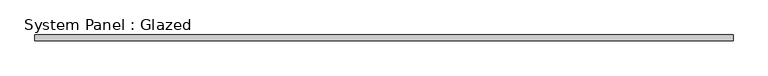
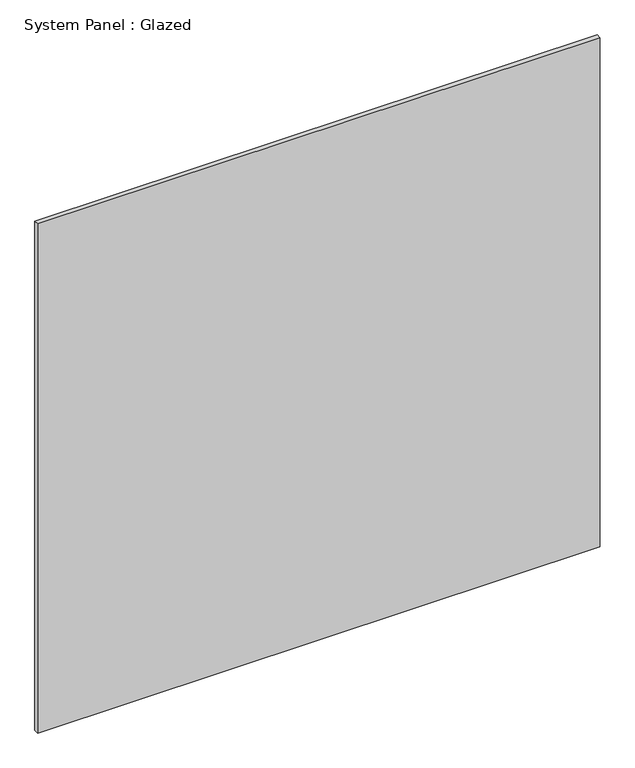
"""IFC4 building model written with IfcOpenShell, lengths in millimetres: plate geometry, System Panel : Glazed."""

from ifc_helpers import new_model, si_unit, origin, origin_with_axes, place, context, project, spatial, polyline, outline, extrude, source, transform, mapped, element, save


def system_panel_glazed_c3829408(model_context):
    return source(origin(), model_context, "Body", "SweptSolid", [
        extrude(outline(polyline([(1526.4620883, 19.05), (-1526.4620883, 19.05), (-1526.4620883, 44.45), (1526.4620883, 44.45), (1526.4620883, 19.05)])), origin_with_axes(), (0.0, 0.0, 1.0), 2921.0),
    ])


if __name__ == "__main__":
    model = new_model("IFC4")
    model_context = context("Model", 3, world=origin())
    ifc_project = project(units=[si_unit("LENGTHUNIT", "METRE", prefix="MILLI")], contexts=[model_context])
    site = spatial("IfcSite", under=ifc_project)
    building = spatial("IfcBuilding", under=site)
    placement = place(None, origin())
    system_panel_glazed_shape = system_panel_glazed_c3829408(model_context)
    element("IfcPlate", 1, ObjectType="System Panel : Glazed", at=placement, inside=building, context=model_context, shape_type="MappedRepresentation", body=[
        mapped(system_panel_glazed_shape, transform((0.0, 0.0, 0.0), x_axis=(1.0, 0.0, 0.0), y_axis=(0.0, 1.0, 0.0), z_axis=(0.0, 0.0, 1.0))),
    ])
    save(model, "model.ifc")

# Revit data of these elements
# Type "System Panel : Glazed"
#   Construction Type Id = "GSP4R"
#   Analytic Construction = "1/8 in Pilkington single glazing"
#   Visual Light Transmittance = 0.9
#   Solar Heat Gain Coefficient = 0.86
#   Heat Transfer Coefficient (U) = 1.18115 BTU/(h·ft²·°F)
#   Define Thermal Properties by = 1
# Element 1 (IfcPlate, "System Panel : Glazed")
#   Materials on its faces: "Glass"
# Materials
#   "Glass": class "Glass", colour RGB 0 128 192, transparency 0.75, Description = "Soda Lime Glass", Cost = 0
